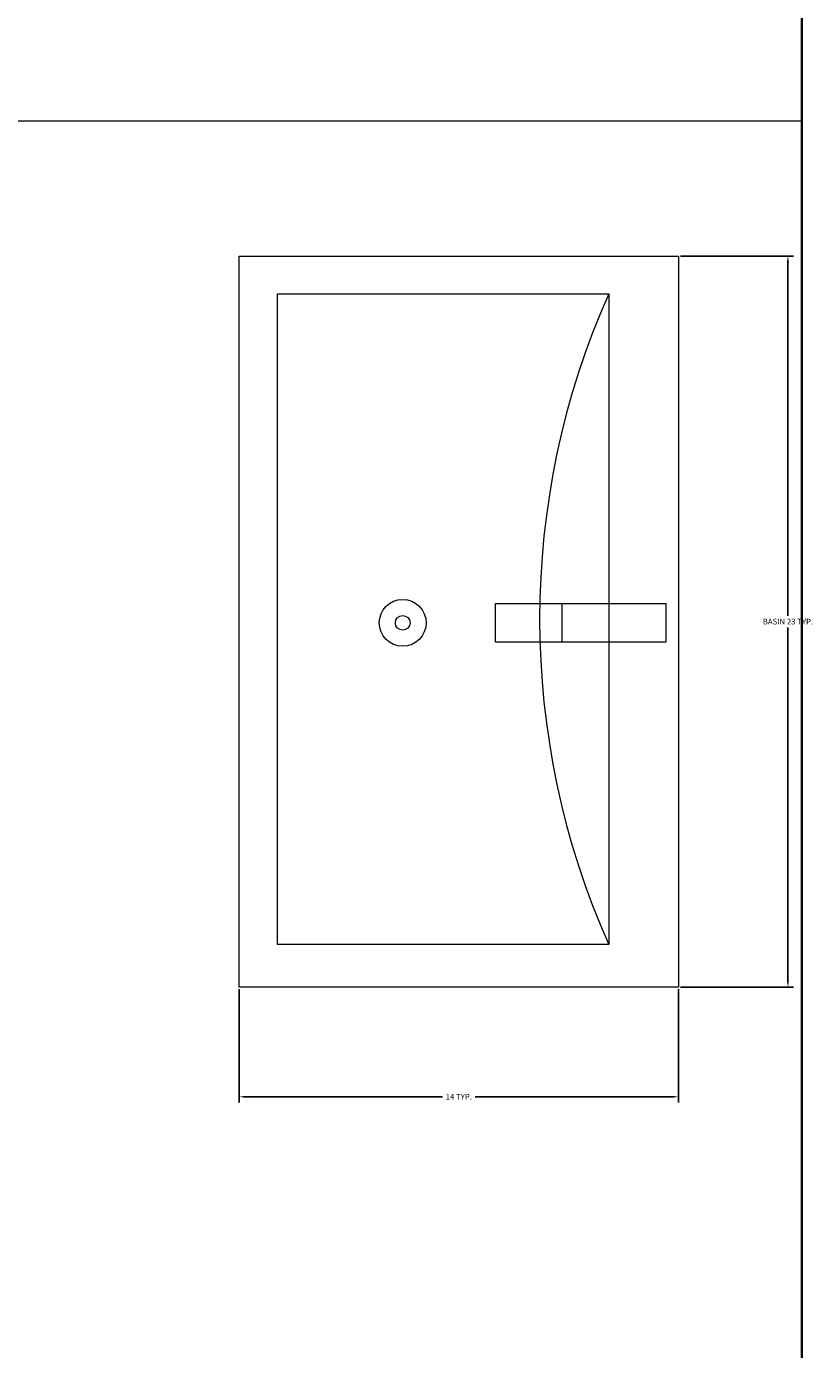
# Model space of a CAD drawing. Units: inches. Extents: x -61 to 1599, y -1316 to 257.
# Tile 174 of 204: x 1351 to 1376, y -684 to -643. Entities that reach past the tile are written whole.
import ezdxf

# ---------------------------------------------------------------- set-up
doc = ezdxf.new("R2010")
doc.units = ezdxf.units.IN
doc.header["$MEASUREMENT"] = 0
for name, color, linetype, lineweight in [('A-ANNO-DIMS', 2, 'Continuous', 18), ('A-FLOR-FIXT', 8, 'Continuous', 18), ('WALLS', 4, 'Continuous', 35)]:
    doc.layers.add(name, color=color, linetype=linetype, lineweight=lineweight)
doc.styles.get("Standard").update_dxf_attribs({"font": 'arial.ttf'})
doc.dimstyles.get("Standard").update_dxf_attribs({"dimtxt": 0.18, "dimasz": 0.18, "dimexe": 0.18, "dimexo": 0.0625, "dimgap": 0.09, "dimtad": 0, "dimtih": 1, "dimtoh": 1, "dimdec": 0, "dimzin": 0, "dimdsep": 46, "dimlunit": 3, "dimtxsty": 'Standard', "dimcen": 0.09, "dimadec": 0, "dimazin": 0, "dimtfac": 1, "dimtdec": 0, "dimtofl": 0, "dimtmove": 0, "dimatfit": 3, "dimfxl": 1, "dimtolj": 1, "dimtzin": 0, "dimarcsym": 0})

# ---------------------------------------------------------------- blocks, each defined once
blk = doc.blocks.new('LAVATORY-WALL')
blk.add_line((10.191, 12.111), (10.191, 10.884))
for points in [[(13.866, 0), (0, 0), (0, 23.069), (13.866, 23.069)], [(13.866, 0), (0, 0), (0, 23.069), (13.866, 23.069)], [(1.203, 1.342), (1.203, 21.884), (11.667, 21.884), (11.667, 1.342)], [(8.089, 10.884), (8.089, 12.111), (13.47, 12.111), (13.47, 10.884)]]:
    blk.add_lwpolyline(points, close=True)
for radius in [0.74, 0.233]:
    blk.add_circle((5.161, 11.497), radius)
blk.add_arc((34.73, 11.613), 25.246, 155.9939, 204.0061)
blk = doc.blocks.new('*D624')
at = {"layer": 'A-ANNO-DIMS', "color": 0, "lineweight": -2, "transparency": 16777216}
for p, q in [((1371.864, -649.913), (1375.442, -649.913)), ((1375.262, -650.093), (1375.262, -661.264)), ((1375.262, -672.802), (1375.262, -661.63)), ((1371.864, -672.982), (1375.442, -672.982))]:
    blk.add_line(p, q, dxfattribs=at)
at = {"layer": 'A-ANNO-DIMS', "color": 0, "transparency": 16777216}
for points in [[(1375.232, -650.093), (1375.292, -650.093), (1375.262, -649.913)], [(1375.232, -672.802), (1375.292, -672.802), (1375.262, -672.982)]]:
    blk.add_solid(points, dxfattribs=at)
at = {"layer": 'DEFPOINTS', "color": 0, "transparency": 16777216}
for p in [(1371.802, -649.913), (1375.262, -649.913), (1371.802, -672.982)]:
    blk.add_point(p, dxfattribs=at)
at = {"layer": 'A-ANNO-DIMS', "color": 0, "transparency": 16777216, "insert": (1375.262, -661.447), "char_height": 0.18, "attachment_point": 5}
blk.add_mtext('\\A1;BASIN 23 TYP.', dxfattribs=at)
blk = doc.blocks.new('*D625')
at = {"layer": 'A-ANNO-DIMS', "color": 0, "lineweight": -2, "transparency": 16777216}
for p, q in [((1357.936, -673.044), (1357.936, -676.622)), ((1371.802, -673.044), (1371.802, -676.622)), ((1358.116, -676.442), (1364.349, -676.442)), ((1371.622, -676.442), (1365.388, -676.442))]:
    blk.add_line(p, q, dxfattribs=at)
at = {"layer": 'A-ANNO-DIMS', "color": 0, "transparency": 16777216}
for points in [[(1358.116, -676.412), (1358.116, -676.472), (1357.936, -676.442)], [(1371.622, -676.412), (1371.622, -676.472), (1371.802, -676.442)]]:
    blk.add_solid(points, dxfattribs=at)
at = {"layer": 'DEFPOINTS', "color": 0, "transparency": 16777216}
for p in [(1357.936, -672.982), (1371.802, -672.982), (1371.802, -676.442)]:
    blk.add_point(p, dxfattribs=at)
at = {"layer": 'A-ANNO-DIMS', "color": 0, "transparency": 16777216, "insert": (1364.869, -676.442), "char_height": 0.18, "attachment_point": 5}
blk.add_mtext('\\A1;14 TYP.', dxfattribs=at)

msp = doc.modelspace()

# ---------------------------------------------------------------- linework, layer by layer
at = {"layer": 'A-FLOR-FIXT'}
msp.add_line((1305.7028, -645.6384), (1375.7028, -645.6384), dxfattribs=at)
at = {"layer": 'WALLS'}
msp.add_line((1375.7028, -621.169), (1375.7028, -729.169), dxfattribs=at)

# ---------------------------------------------------------------- block references
at = {"layer": 'A-FLOR-FIXT'}
msp.add_blockref('LAVATORY-WALL', (1357.936, -672.9821), dxfattribs=at)

# ---------------------------------------------------------------- dimensions: what is measured, and where the dimension line sits
at = {"layer": 'A-ANNO-DIMS'}
dim = msp.add_linear_dim(base=(1375.262, -649.9127), p1=(1371.8016, -672.9818), p2=(1371.8016, -649.9127), angle=90, text='BASIN <> TYP.', dimstyle='Standard', override={"dimdec": 0, "dimlfac": 1, "dimrnd": 0, "dimzin": 0, "dimdsep": 46, "dimlunit": 2}, dxfattribs=at)
dim.commit()
dim.dimension.update_dxf_attribs({"geometry": '*D624', "text_midpoint": (1375.262, -661.4473)})
dim = msp.add_linear_dim(base=(1371.8016, -676.4422), p1=(1357.9359, -672.9818), p2=(1371.8016, -672.9818), text='<> TYP.', dimstyle='Standard', override={"dimdec": 0, "dimlfac": 1, "dimrnd": 0, "dimzin": 0, "dimdsep": 46, "dimlunit": 2}, dxfattribs=at)
dim.commit()
dim.dimension.update_dxf_attribs({"geometry": '*D625', "text_midpoint": (1364.8688, -676.4422)})

doc.saveas('drawing.dxf')
